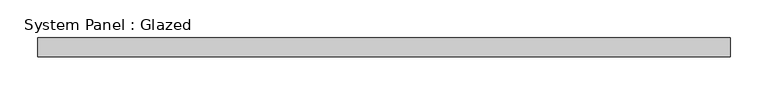
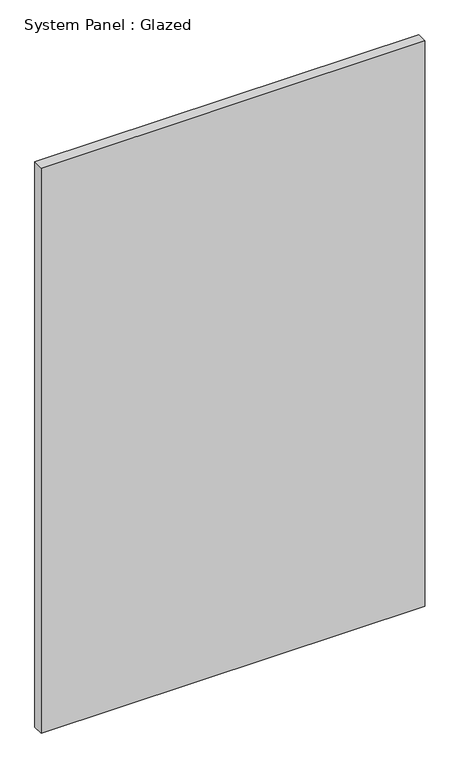
"""IFC4 building model written with IfcOpenShell, lengths in millimetres: plate geometry, System Panel : Glazed."""

from ifc_helpers import new_model, si_unit, origin, origin_with_axes, place, context, project, spatial, polyline, outline, extrude, source, transform, mapped, element, save


def system_panel_glazed_9eaa7c8f(model_context):
    return source(origin(), model_context, "Body", "SweptSolid", [
        extrude(outline(polyline([(460.375, 19.05), (-460.375, 19.05), (-460.375, 44.45), (460.375, 44.45), (460.375, 19.05)])), origin_with_axes(), (0.0, 0.0, 1.0), 1433.9513331),
    ])


if __name__ == "__main__":
    model = new_model("IFC4")
    model_context = context("Model", 3, world=origin())
    ifc_project = project(units=[si_unit("LENGTHUNIT", "METRE", prefix="MILLI")], contexts=[model_context])
    site = spatial("IfcSite", under=ifc_project)
    building = spatial("IfcBuilding", under=site)
    placement = place(None, origin())
    system_panel_glazed_shape = system_panel_glazed_9eaa7c8f(model_context)
    element("IfcPlate", 1, ObjectType="System Panel : Glazed", at=placement, inside=building, context=model_context, shape_type="MappedRepresentation", body=[
        mapped(system_panel_glazed_shape, transform((0.0, 0.0, 0.0), x_axis=(1.0, 0.0, 0.0), y_axis=(0.0, 1.0, 0.0), z_axis=(0.0, 0.0, 1.0))),
    ])
    save(model, "model.ifc")

# Revit data of these elements
# Type "System Panel : Glazed"
#   Construction Type Id = "GSP4R"
#   Analytic Construction = "1/8 in Pilkington single glazing"
#   Visual Light Transmittance = 0.9
#   Solar Heat Gain Coefficient = 0.86
#   Heat Transfer Coefficient (U) = 1.18115 BTU/(h·ft²·°F)
#   Define Thermal Properties by = 1
# Element 1 (IfcPlate, "System Panel : Glazed")
#   Materials on its faces: "Glass"
# Materials
#   "Glass": class "Glass", colour RGB 0 128 192, transparency 0.75, Description = "Soda Lime Glass", Cost = 0
